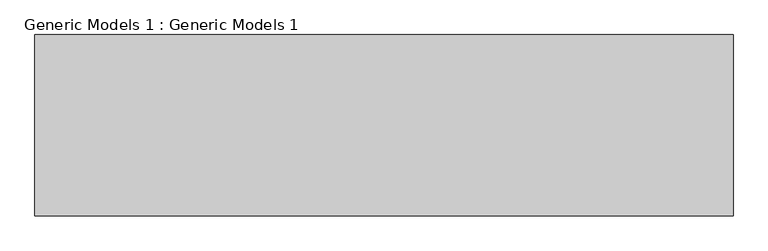
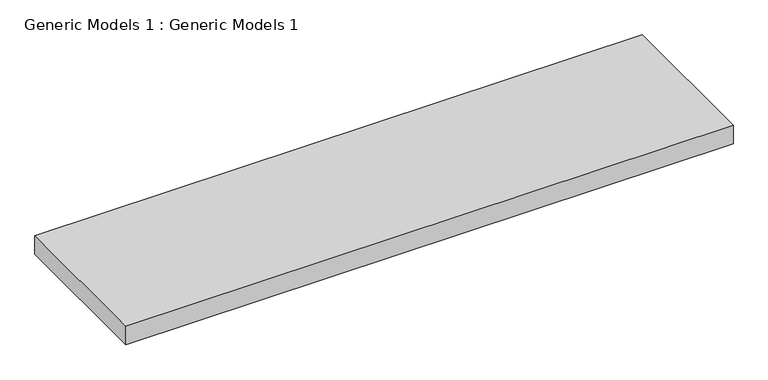
"""IFC4 building model written with IfcOpenShell, lengths in millimetres: proxy geometry, Generic Models 1 : Generic Models 1."""

from ifc_helpers import new_model, si_unit, origin, origin_with_axes, place, context, project, spatial, polyline, outline, extrude, source, transform, mapped, element, save


def generic_models_1_generic_models_1_1e977ea9(model_context):
    return source(origin(), model_context, "Body", "SweptSolid", [
        extrude(outline(polyline([(-5613.1530968, -12966.858307), (-5613.1530968, -15458.6370893), (-15214.3530968, -15458.6370893), (-15214.3530968, -12966.858307), (-5613.1530968, -12966.858307)])), origin_with_axes(), (0.0, 0.0, 1.0), 304.8),
    ])


if __name__ == "__main__":
    model = new_model("IFC4")
    model_context = context("Model", 3, world=origin())
    ifc_project = project(units=[si_unit("LENGTHUNIT", "METRE", prefix="MILLI")], contexts=[model_context])
    site = spatial("IfcSite", under=ifc_project)
    building = spatial("IfcBuilding", under=site)
    placement = place(None, origin())
    generic_models_1_generic_models_1_shape = generic_models_1_generic_models_1_1e977ea9(model_context)
    element("IfcBuildingElementProxy", 1, Name="Generic Models 1 : Generic Models 1", ObjectType="Generic Models 1 : Generic Models 1", at=placement, inside=building, context=model_context, shape_type="MappedRepresentation", body=[
        mapped(generic_models_1_generic_models_1_shape, transform((0.0, 0.0, 0.0), x_axis=(1.0, 0.0, 0.0), y_axis=(0.0, 1.0, 0.0), z_axis=(0.0, 0.0, 1.0))),
    ])
    save(model, "model.ifc")
